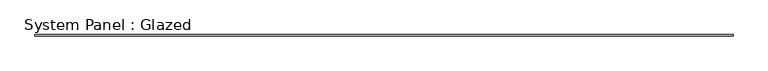
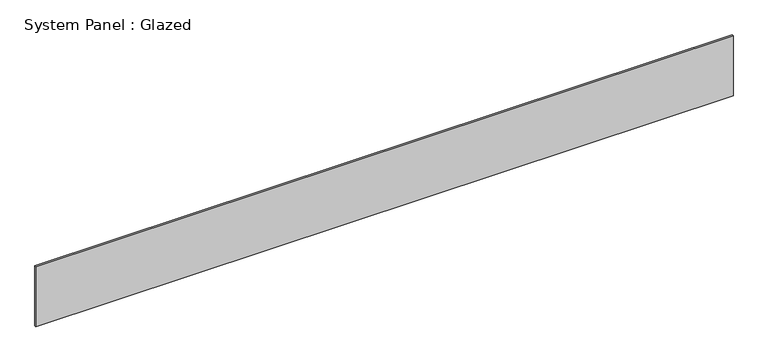
"""IFC4 building model written with IfcOpenShell, lengths in millimetres: plate geometry, System Panel : Glazed."""

from ifc_helpers import new_model, si_unit, origin, origin_with_axes, place, context, project, spatial, polyline, outline, extrude, source, transform, mapped, element, save


def system_panel_glazed_56f52ef6(model_context):
    return source(origin(), model_context, "Body", "SweptSolid", [
        extrude(outline(polyline([(6350.1330359, 19.05), (-6350.1330359, 19.05), (-6350.1330359, 44.45), (6350.1330359, 44.45), (6350.1330359, 19.05)])), origin_with_axes(), (0.0, 0.0, 1.0), 1155.7),
    ])


if __name__ == "__main__":
    model = new_model("IFC4")
    model_context = context("Model", 3, world=origin())
    ifc_project = project(units=[si_unit("LENGTHUNIT", "METRE", prefix="MILLI")], contexts=[model_context])
    site = spatial("IfcSite", under=ifc_project)
    building = spatial("IfcBuilding", under=site)
    placement = place(None, origin())
    system_panel_glazed_shape = system_panel_glazed_56f52ef6(model_context)
    element("IfcPlate", 1, ObjectType="System Panel : Glazed", at=placement, inside=building, context=model_context, shape_type="MappedRepresentation", body=[
        mapped(system_panel_glazed_shape, transform((0.0, 0.0, 0.0), x_axis=(1.0, 0.0, 0.0), y_axis=(0.0, 1.0, 0.0), z_axis=(0.0, 0.0, 1.0))),
    ])
    save(model, "model.ifc")

# Revit data of these elements
# Type "System Panel : Glazed"
#   Construction Type Id = "GSP4R"
#   Analytic Construction = "1/8 in Pilkington single glazing"
#   Visual Light Transmittance = 0.9
#   Solar Heat Gain Coefficient = 0.86
#   Heat Transfer Coefficient (U) = 1.18115 BTU/(h·ft²·°F)
# Element 1 (IfcPlate, "System Panel : Glazed")
#   Materials on its faces: "Glass"
# Materials
#   "Glass": class "Glass", colour RGB 0 128 192, transparency 0.75, Description = "Soda Lime Glass", Cost = 0
